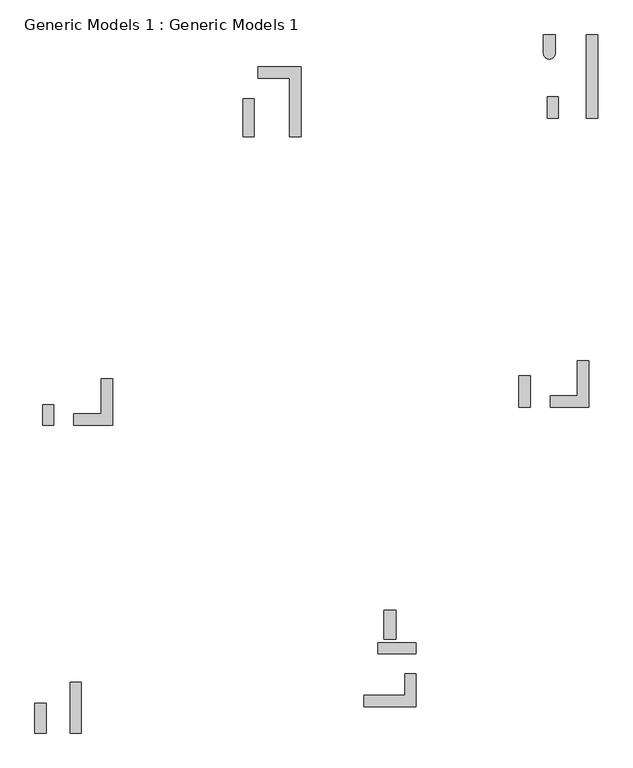
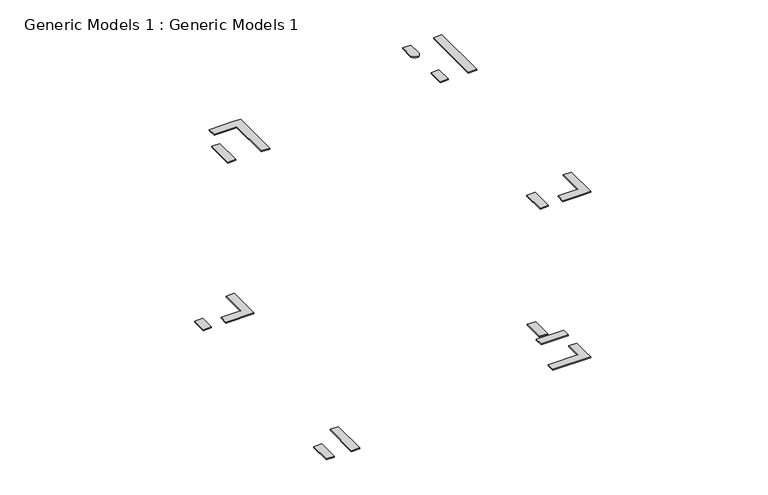
"""IFC4 building model written with IfcOpenShell, lengths in millimetres: proxy geometry, Generic Models 1 : Generic Models 1."""

from ifc_helpers import new_model, si_unit, point, frame, frame_2d, origin, place, context, project, spatial, polyline, circle_curve, trimmed, segment, composite_curve, outline, extrude, source, transform, mapped, element, save


def generic_models_1_generic_models_1_5b52610c(model_context):
    return source(origin(), model_context, "Body", "SweptSolid", [
        extrude(outline(polyline([(-7140.2172689, 59014.1988652), (-7140.2172689, 56341.0496151), (-7730.610903, 56341.0496151), (-7730.610903, 59014.1988652), (-7140.2172689, 59014.1988652)])), frame((0.0, 0.0, 1219.2), z_axis=(0.0, 0.0, 1.0), x_axis=(1.0, 0.0, 0.0)), (0.0, 0.0, 1.0), 76.2),
        extrude(outline(polyline([(-8970.9756011, 57890.7636407), (-8970.9756011, 56341.0496151), (-9569.1368296, 56341.0496151), (-9569.1368296, 57890.7636407), (-8970.9756011, 57890.7636407)])), frame((0.0, 0.0, 1219.2), z_axis=(0.0, 0.0, 1.0), x_axis=(1.0, 0.0, 0.0)), (0.0, 0.0, 1.0), 76.2),
        extrude(outline(polyline([(10401.103694, 61079.901994), (10401.103694, 60494.9153212), (8411.6840136, 60494.9153212), (8411.6840136, 61079.901994), (10401.103694, 61079.901994)])), frame((0.0, 0.0, 1219.2), z_axis=(0.0, 0.0, 1.0), x_axis=(1.0, 0.0, 0.0)), (0.0, 0.0, 1.0), 76.2),
        extrude(outline(polyline([(9809.1108422, 58324.2747834), (9809.1108422, 59455.9463014), (10401.103694, 59455.9463014), (10401.103694, 58324.2747834), (10401.103694, 57707.6433045), (7664.8933567, 57707.6433045), (7664.8933567, 58324.2747834), (9809.1108422, 58324.2747834)])), frame((0.0, 0.0, 1219.2), z_axis=(0.0, 0.0, 1.0), x_axis=(1.0, 0.0, 0.0)), (0.0, 0.0, 1.0), 76.2),
        extrude(outline(polyline([(16395.6982041, 75047.0452261), (16395.6982041, 73398.3878957), (15788.8222029, 73398.3878957), (15788.8222029, 75047.0452261), (16395.6982041, 75047.0452261)])), frame((0.0, 0.0, 1219.2), z_axis=(0.0, 0.0, 1.0), x_axis=(1.0, 0.0, 0.0)), (0.0, 0.0, 1.0), 76.2),
        extrude(outline(polyline([(19454.7969726, 75831.7078957), (19454.7969726, 73398.3878957), (18860.5765423, 73398.3878957), (17438.1765423, 73398.3878957), (17438.1765423, 73995.2878957), (18860.5765423, 73995.2878957), (18860.5765423, 75831.7078957), (19454.7969726, 75831.7078957)])), frame((0.0, 0.0, 1219.2), z_axis=(0.0, 0.0, 1.0), x_axis=(1.0, 0.0, 0.0)), (0.0, 0.0, 1.0), 76.2),
        extrude(outline(polyline([(19934.5396703, 92893.9205337), (19934.5396703, 88524.4937403), (19334.7658915, 88524.4937403), (19334.7658915, 92893.9205337), (19934.5396703, 92893.9205337)])), frame((0.0, 0.0, 1219.2), z_axis=(0.0, 0.0, 1.0), x_axis=(1.0, 0.0, 0.0)), (0.0, 0.0, 1.0), 76.2),
        extrude(outline(polyline([(17853.4882601, 89661.2963913), (17853.4882601, 88524.4937403), (17293.2569726, 88524.4937403), (17293.2569726, 89661.2963913), (17853.4882601, 89661.2963913)])), frame((0.0, 0.0, 1219.2), z_axis=(0.0, 0.0, 1.0), x_axis=(1.0, 0.0, 0.0)), (0.0, 0.0, 1.0), 76.2),
        extrude(outline(polyline([(1909.0057832, 89553.6416254), (1909.0057832, 87568.8962935), (1330.705001, 87568.8962935), (1330.705001, 89553.6416254), (1909.0057832, 89553.6416254)])), frame((0.0, 0.0, 1219.2), z_axis=(0.0, 0.0, 1.0), x_axis=(1.0, 0.0, 0.0)), (0.0, 0.0, 1.0), 76.2),
        extrude(outline(polyline([(3765.5026816, 87568.8962935), (3765.5026816, 90633.3997304), (2116.5336072, 90633.3997304), (2116.5336072, 91223.2213985), (3765.5026816, 91223.2213985), (4376.8368387, 91223.2213985), (4376.8368387, 87568.8962935), (3765.5026816, 87568.8962935)])), frame((0.0, 0.0, 1219.2), z_axis=(0.0, 0.0, 1.0), x_axis=(1.0, 0.0, 0.0)), (0.0, 0.0, 1.0), 76.2),
        extrude(outline(polyline([(-8572.4460585, 73532.0527724), (-8572.4460585, 72458.9027724), (-9163.1131346, 72458.9027724), (-9163.1131346, 73532.0527724), (-8572.4460585, 73532.0527724)])), frame((0.0, 0.0, 1219.2), z_axis=(0.0, 0.0, 1.0), x_axis=(1.0, 0.0, 0.0)), (0.0, 0.0, 1.0), 76.2),
        extrude(outline(polyline([(-6099.6862628, 73054.8296735), (-6099.6862628, 74901.1127724), (-5492.8131346, 74901.1127724), (-5492.8131346, 73054.8296735), (-5492.8131346, 72458.9027724), (-7532.5316906, 72458.9027724), (-7532.5316906, 73054.8296735), (-6099.6862628, 73054.8296735)])), frame((0.0, 0.0, 1219.2), z_axis=(0.0, 0.0, 1.0), x_axis=(1.0, 0.0, 0.0)), (0.0, 0.0, 1.0), 76.2),
        extrude(outline(polyline([(9346.6401818, 62781.701994), (9346.6401818, 61253.637994), (8730.5821922, 61253.637994), (8730.5821922, 62781.701994), (9346.6401818, 62781.701994)])), frame((0.0, 0.0, 1219.2), z_axis=(0.0, 0.0, 1.0), x_axis=(1.0, 0.0, 0.0)), (0.0, 0.0, 1.0), 76.2),
        extrude(outline(composite_curve([segment(trimmed(circle_curve(frame_2d((17385.4647661, 91928.7205337)), 301.4922065), [point((17686.9569726, 91928.7205337))], [point((17083.9725595, 91928.7205337))], False, "CARTESIAN"), True, "CONTINUOUS"), segment(polyline([(17083.9725595, 91928.7205337), (17083.9725595, 92893.9205337), (17686.9569726, 92893.9205337), (17686.9569726, 91928.7205337)]), True, "CONTINUOUS")], self_intersect=False)), frame((0.0, 0.0, 1219.2), z_axis=(0.0, 0.0, 1.0), x_axis=(1.0, 0.0, 0.0)), (0.0, 0.0, 1.0), 76.2),
    ])


if __name__ == "__main__":
    model = new_model("IFC4")
    model_context = context("Model", 3, world=origin())
    ifc_project = project(units=[si_unit("LENGTHUNIT", "METRE", prefix="MILLI")], contexts=[model_context])
    site = spatial("IfcSite", under=ifc_project)
    building = spatial("IfcBuilding", under=site)
    placement = place(None, origin())
    generic_models_1_generic_models_1_shape = generic_models_1_generic_models_1_5b52610c(model_context)
    element("IfcBuildingElementProxy", 1, Name="Generic Models 1 : Generic Models 1", ObjectType="Generic Models 1 : Generic Models 1", at=placement, inside=building, context=model_context, shape_type="MappedRepresentation", body=[
        mapped(generic_models_1_generic_models_1_shape, transform((0.0, 0.0, 0.0), x_axis=(1.0, 0.0, 0.0), y_axis=(0.0, 1.0, 0.0), z_axis=(0.0, 0.0, 1.0))),
    ])
    save(model, "model.ifc")

# Revit data of these elements
# Element 1 (IfcBuildingElementProxy, "Generic Models 1 : Generic Models 1")
#   Materials on its faces: "HALL"
# Materials
#   "HALL": class "Generic", colour RGB 120 120 120, transparency 0, Cost = 0
